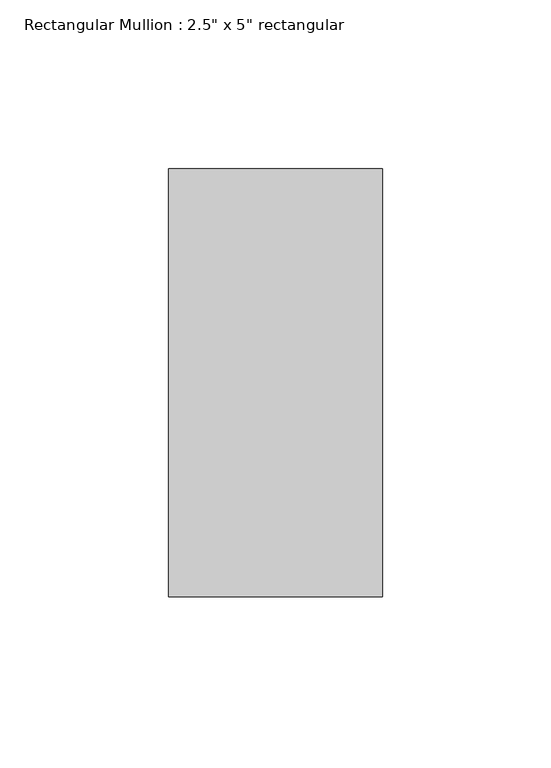
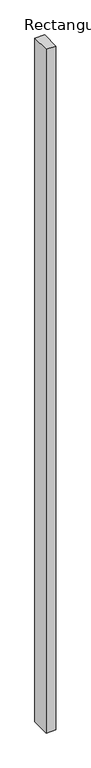
"""IFC4 building model written with IfcOpenShell, lengths in millimetres: member geometry."""

from ifc_helpers import new_model, si_unit, frame, origin, place, context, project, spatial, polyline, outline, extrude, source, transform, mapped, element, save


def member_01548017(model_context):
    return source(origin(), model_context, "Body", "SweptSolid", [
        extrude(outline(polyline([(0.0, 63.5), (0.0, -63.5), (-63.5, -63.5), (-63.5, 63.5), (0.0, 63.5)])), frame((0.0, 0.0, -4699.0), z_axis=(0.0, 0.0, 1.0), x_axis=(1.0, 0.0, 0.0)), (0.0, 0.0, 1.0), 4699.0),
    ])


if __name__ == "__main__":
    model = new_model("IFC4")
    model_context = context("Model", 3, world=origin())
    ifc_project = project(units=[si_unit("LENGTHUNIT", "METRE", prefix="MILLI")], contexts=[model_context])
    site = spatial("IfcSite", under=ifc_project)
    building = spatial("IfcBuilding", under=site)
    placement = place(None, origin())
    member_shape = member_01548017(model_context)
    element("IfcMember", 1, ObjectType="Rectangular Mullion : 2.5\" x 5\" rectangular", at=placement, inside=building, context=model_context, shape_type="MappedRepresentation", body=[
        mapped(member_shape, transform((0.0, 0.0, 0.0), x_axis=(1.0, 0.0, 0.0), y_axis=(0.0, 1.0, 0.0), z_axis=(0.0, 0.0, 1.0))),
    ])
    save(model, "model.ifc")

# Revit data of these elements
# Type "Rectangular Mullion : 2.5\" x 5\" rectangular"
#   built-in parameter 1007304 = 0.416667 (stored number, unit not read)
#   built-in parameter 1007301 = 0.104167 (stored number, unit not read)
#   built-in parameter 1007300 = 0.104167 (stored number, unit not read)
# Element 1 (IfcMember, "Rectangular Mullion : 2.5\" x 5\" rectangular")
#   Materials on its faces: "Aluminum"
# Materials
#   "Aluminum": class "Metal", colour RGB 247 247 247, transparency 0, Description = "Aluminum 6061", Cost = 0
